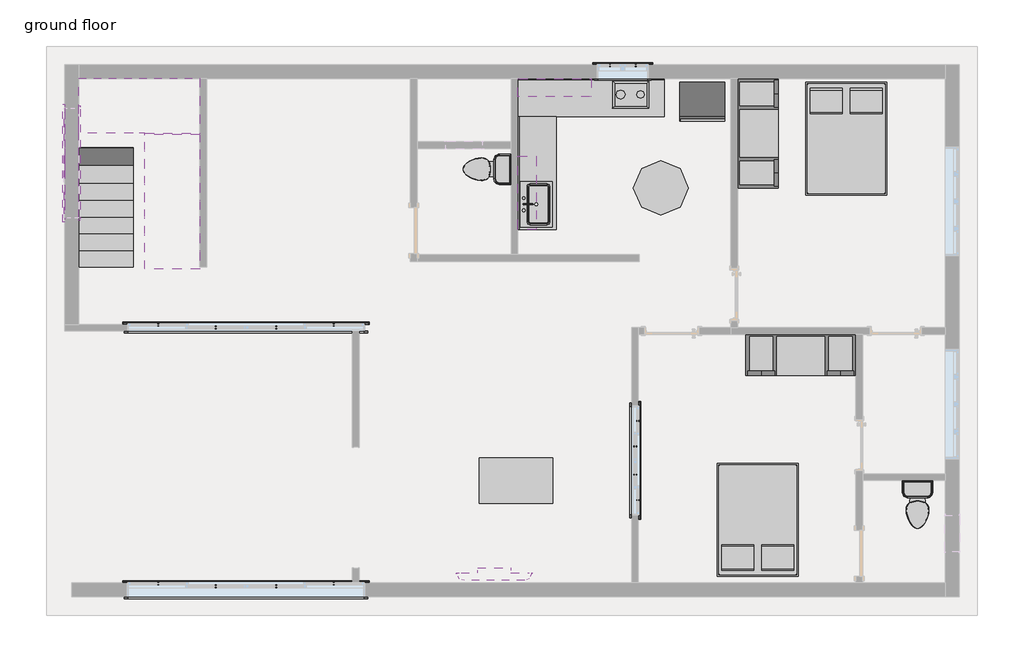
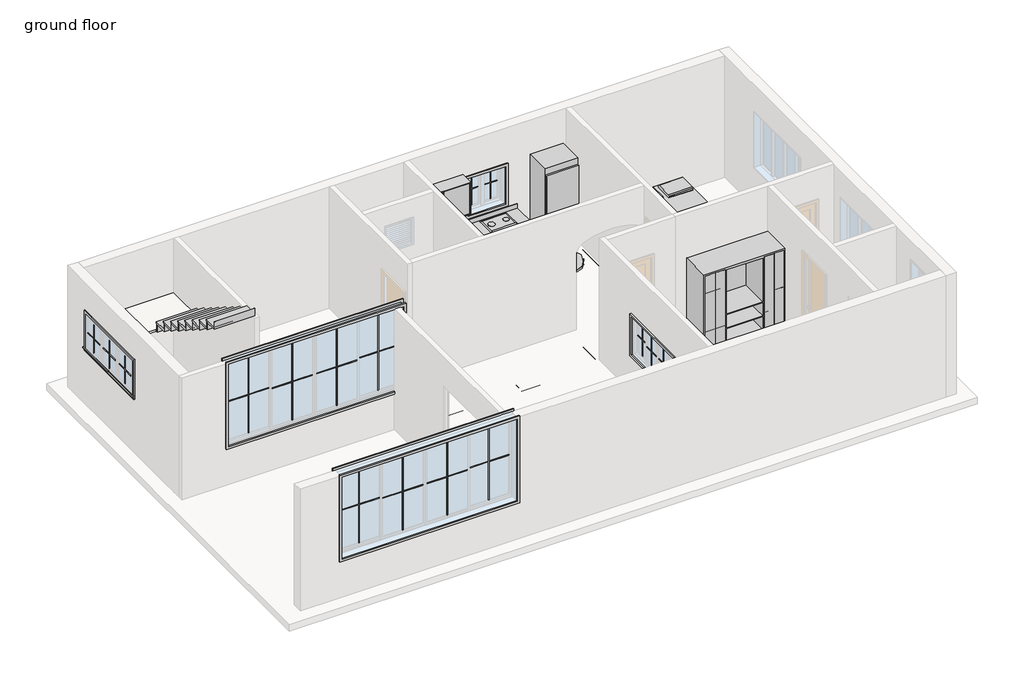
# One storey, part 2 of 2: 30 proxies, 15 furniture elements, 9 beams, 3 flow terminals, 2 stair flights, 1 slab.
"""IFC4 building model written with IfcOpenShell, lengths in millimetres."""

from ifc_helpers import new_model, si_unit, frame, origin, place, context, project, spatial, polyline, outline, extrude, faceted_brep, transform, mapped, element, save
from components import proxy_3c1fa1d0, proxy_caef4acf, muntin_pattern_2x2_muntin_pattern_2x2_31a16349, muntin_pattern_2x2_muntin_pattern_2x2_a56fcb99, muntin_pattern_2x2_muntin_pattern_2x2_c58f38d7, muntin_pattern_2x2_muntin_pattern_2x2_b3fe6957, muntin_pattern_2x2_muntin_pattern_2x2_3e0ecaf2, muntin_pattern_2x2_muntin_pattern_2x2_51cb8927, proxy_19935bb1, trim_window_exterior_flat_with_sill_3c945769, trim_window_exterior_flat_with_sill_7b949e88, trim_window_exterior_flat_with_sill_41619996, trim_window_exterior_flat_with_sill_170b7f0e, trim_window_interior_flat_picture_frame_0edfbaa2, trim_window_interior_flat_picture_frame_687edbe0, trim_window_interior_flat_picture_frame_51c85655, trim_window_interior_flat_picture_frame_cc79b2fe, flow_terminal_4d548711, toilet_domestic_3d_toilet_domestic_3d_ba6479b0, toilet_domestic_3d_toilet_domestic_3d_30431060, furniture_f87f75a4, furniture_97fe820d, furniture_b58f7881, furniture_deb1c5d1, furniture_078eb3f3, furniture_88072bd9, furniture_0b81fedb, furniture_acc2807d, furniture_52f35bf4, furniture_f491f192, non_monolithic_landing_2b816123, stair_flight_0432408d, stair_flight_b9007331

model = new_model("IFC4")

# Units and contexts
model_context = context("Model", 3, world=origin())
ifc_project = project(units=[si_unit("LENGTHUNIT", "METRE", prefix="MILLI")], contexts=[model_context])

# Site, building, storey
site = spatial("IfcSite", under=ifc_project)
building = spatial("IfcBuilding", under=site)
storey = spatial("IfcBuildingStorey", under=building, Name="ground floor", Elevation=609.6)

# Beams
placement = place(None, origin())
element("IfcBeam", 1, ObjectType="Concrete-Rectangular Beam", at=placement, inside=storey, context=model_context, shape_type="Brep", body=[
    faceted_brep([(-12643.368339, 9510.993496, 609.6), (-12643.368339, 9282.393496, 609.6), (-10681.218339, 9282.393496, 609.6), (-10452.618339, 9282.393496, 609.6), (-7176.018339, 9282.393496, 609.6), (-6947.418339, 9282.393496, 609.6), (-5499.618339, 9282.393496, 609.6), (-5271.018339, 9282.393496, 609.6), (-3492.916739, 9282.393496, 609.6), (-3264.316739, 9282.393496, 609.6), (-1842.018339, 9282.393496, 609.6), (-1613.418339, 9282.393496, 609.6), (1790.181661, 9282.393496, 609.6), (1790.181661, 9510.993496, 609.6), (-1575.318339, 9510.993496, 609.6), (-1575.318339, 9320.493496, 609.6), (-1880.118339, 9320.493496, 609.6), (-1880.118339, 9510.993496, 609.6), (-6909.318339, 9510.993496, 609.6), (-6909.318339, 9320.493496, 609.6), (-7214.118339, 9320.493496, 609.6), (-7214.118339, 9510.993496, 609.6), (-10414.518339, 9510.993496, 609.6), (-10414.518339, 9320.493496, 609.6), (-10719.318339, 9320.493496, 609.6), (-10719.318339, 9510.993496, 609.6), (-12643.368339, 9282.393496, 304.8), (-10681.218339, 9282.393496, 304.8), (-10452.618339, 9282.393496, 304.8), (-7176.018339, 9282.393496, 304.8), (-6947.418339, 9282.393496, 304.8), (-5499.618339, 9282.393496, 304.8), (-5271.018339, 9282.393496, 304.8), (-3492.916739, 9282.393496, 304.8), (-3264.316739, 9282.393496, 304.8), (-1842.018339, 9282.393496, 304.8), (-1613.418339, 9282.393496, 304.8), (1790.181661, 9282.393496, 304.8), (-12643.368339, 9510.993496, 304.8), (-10719.318339, 9510.993496, 304.8), (-10719.318339, 9320.493496, 304.8), (-10414.518339, 9320.493496, 304.8), (-10414.518339, 9510.993496, 304.8), (-7214.118339, 9510.993496, 304.8), (-7214.118339, 9320.493496, 304.8), (-6909.318339, 9320.493496, 304.8), (-6909.318339, 9510.993496, 304.8), (-1880.118339, 9510.993496, 304.8), (-1880.118339, 9320.493496, 304.8), (-1575.318339, 9320.493496, 304.8), (-1575.318339, 9510.993496, 304.8), (1790.181661, 9510.993496, 304.8)], [[[0, 1, 2, 3, 4, 5, 6, 7, 8, 9, 10, 11, 12, 13, 14, 15, 16, 17, 18, 19, 20, 21, 22, 23, 24, 25]], [[1, 26, 27, 28, 29, 30, 31, 32, 33, 34, 35, 36, 37, 12, 11, 10, 9, 8, 7, 6, 5, 4, 3, 2]], [[26, 38, 39, 40, 41, 42, 43, 44, 45, 46, 47, 48, 49, 50, 51, 37, 36, 35, 34, 33, 32, 31, 30, 29, 28, 27]], [[13, 51, 50, 14]], [[1, 0, 38, 26]], [[13, 12, 37, 51]], [[41, 23, 22, 42]], [[23, 41, 40, 24]], [[24, 40, 39, 25]], [[45, 19, 18, 46]], [[19, 45, 44, 20]], [[20, 44, 43, 21]], [[49, 15, 14, 50]], [[15, 49, 48, 16]], [[16, 48, 47, 17]], [[38, 0, 25, 39]], [[42, 22, 21, 43]], [[46, 18, 17, 47]]]),
])
element("IfcBeam", 2, ObjectType="Concrete-Rectangular Beam", at=placement, inside=storey, context=model_context, shape_type="Brep", body=[
    faceted_brep([(1790.181661, 913.093496, 609.6), (2018.781661, 913.093496, 609.6), (2018.781661, 4958.043496, 609.6), (1790.181661, 4958.043496, 609.6), (1790.181661, 2792.693496, 609.6), (1790.181661, 2564.093496, 609.6), (1790.181661, 913.093496, 304.8), (1790.181661, 4958.043496, 304.8), (1790.181661, 2792.693496, 304.8), (1790.181661, 2564.093496, 304.8), (2018.781661, 913.093496, 304.8), (2018.781661, 4958.043496, 304.8)], [[[0, 1, 2, 3, 4, 5]], [[6, 0, 5, 4, 3, 7, 8, 9]], [[10, 6, 9, 8, 7, 11]], [[1, 10, 11, 2]], [[1, 0, 6, 10]], [[3, 2, 11, 7]]]),
    faceted_brep([(1790.181661, 9244.293496, 609.6), (2018.781661, 9244.293496, 609.6), (2018.781661, 9244.293496, 304.8), (1790.181661, 9244.293496, 304.8), (2018.781661, 5262.843496, 609.6), (1790.181661, 5262.843496, 609.6), (1790.181661, 5262.843496, 304.8), (2018.781661, 5262.843496, 304.8), (1790.181661, 6443.943496, 609.6), (1790.181661, 6215.343496, 609.6), (1790.181661, 6443.943496, 304.8), (1790.181661, 6215.343496, 304.8)], [[[0, 1, 2, 3]], [[4, 5, 6, 7]], [[1, 0, 8, 9, 5, 4]], [[0, 3, 10, 11, 6, 5, 9, 8]], [[3, 2, 7, 6, 11, 10]], [[2, 1, 4, 7]]]),
])
element("IfcBeam", 3, ObjectType="Concrete-Rectangular Beam", at=placement, inside=storey, context=model_context, shape_type="SweptSolid", body=[
    extrude(outline(polyline([(-6947.418339, 8094.943496), (-6947.418339, 8323.543496), (-5499.618339, 8323.543496), (-5499.618339, 8094.943496), (-6947.418339, 8094.943496)])), frame((0.0, 0.0, 304.8), z_axis=(0.0, 0.0, 1.0), x_axis=(1.0, 0.0, 0.0)), (0.0, 0.0, 1.0), 304.8),
])
element("IfcBeam", 4, ObjectType="Concrete-Rectangular Beam", at=placement, inside=storey, context=model_context, shape_type="Brep", body=[
    faceted_brep([(-6947.418339, 6443.943496, 609.6), (-6947.418339, 6215.343496, 609.6), (-5499.618339, 6215.343496, 609.6), (-5499.618339, 6443.943496, 609.6), (-6947.418339, 6215.343496, 304.8), (-5499.618339, 6215.343496, 304.8), (-6947.418339, 6443.943496, 304.8), (-5499.618339, 6443.943496, 304.8)], [[[0, 1, 2, 3]], [[1, 4, 5, 2]], [[4, 6, 7, 5]], [[6, 0, 3, 7]], [[1, 0, 6, 4]], [[3, 2, 5, 7]]]),
    faceted_brep([(1790.181661, 6443.943496, 609.6), (1790.181661, 6215.343496, 609.6), (1790.181661, 6215.343496, 304.8), (1790.181661, 6443.943496, 304.8), (-5271.018339, 6215.343496, 609.6), (-5271.018339, 6443.943496, 609.6), (-5271.018339, 6443.943496, 304.8), (-5271.018339, 6215.343496, 304.8), (-1613.418339, 6443.943496, 609.6), (-1842.018339, 6443.943496, 609.6), (-3264.316739, 6443.943496, 609.6), (-3492.916739, 6443.943496, 609.6), (-3492.916739, 6215.343496, 609.6), (-3264.316739, 6215.343496, 609.6), (-1842.018339, 6215.343496, 609.6), (-1613.418339, 6215.343496, 609.6), (-3492.916739, 6215.343496, 304.8), (-3264.316739, 6215.343496, 304.8), (-1842.018339, 6215.343496, 304.8), (-1613.418339, 6215.343496, 304.8), (-3492.916739, 6443.943496, 304.8), (-3264.316739, 6443.943496, 304.8), (-1842.018339, 6443.943496, 304.8), (-1613.418339, 6443.943496, 304.8)], [[[0, 1, 2, 3]], [[4, 5, 6, 7]], [[1, 0, 8, 9, 10, 11, 5, 4, 12, 13, 14, 15]], [[2, 1, 15, 14, 13, 12, 4, 7, 16, 17, 18, 19]], [[3, 2, 19, 18, 17, 16, 7, 6, 20, 21, 22, 23]], [[0, 3, 23, 22, 21, 20, 6, 5, 11, 10, 9, 8]]]),
])
element("IfcBeam", 5, ObjectType="Concrete-Rectangular Beam", at=placement, inside=storey, context=model_context, shape_type="Brep", body=[
    faceted_brep([(-1842.018339, 913.093496, 609.6), (-1613.418339, 913.093496, 609.6), (-1613.418339, 4996.143496, 609.6), (-1613.418339, 5224.743496, 609.6), (-1613.418339, 6215.343496, 609.6), (-1842.018339, 6215.343496, 609.6), (-1842.018339, 5281.893496, 609.6), (-1784.868339, 5281.893496, 609.6), (-1784.868339, 5053.293496, 609.6), (-1842.018339, 5053.293496, 609.6), (-1842.018339, 4996.143496, 609.6), (-1842.018339, 913.093496, 304.8), (-1842.018339, 5053.293496, 304.8), (-1842.018339, 4996.143496, 304.8), (-1613.418339, 913.093496, 304.8), (-1784.868339, 5053.293496, 304.8), (-1784.868339, 5281.893496, 304.8), (-1842.018339, 5281.893496, 304.8), (-1842.018339, 6215.343496, 304.8), (-1613.418339, 6215.343496, 304.8), (-1613.418339, 5224.743496, 304.8), (-1613.418339, 4996.143496, 304.8)], [[[0, 1, 2, 3, 4, 5, 6, 7, 8, 9, 10]], [[11, 0, 10, 9, 12, 13]], [[14, 11, 13, 12, 15, 16, 17, 18, 19, 20, 21]], [[1, 14, 21, 20, 19, 4, 3, 2]], [[1, 0, 11, 14]], [[8, 15, 12, 9]], [[16, 7, 6, 17]], [[7, 16, 15, 8]], [[17, 6, 5, 18]], [[5, 4, 19, 18]]]),
    faceted_brep([(-1842.018339, 9282.393496, 609.6), (-1613.418339, 9282.393496, 609.6), (-1613.418339, 9282.393496, 304.8), (-1842.018339, 9282.393496, 304.8), (-1613.418339, 6443.943496, 609.6), (-1842.018339, 6443.943496, 609.6), (-1842.018339, 6443.943496, 304.8), (-1613.418339, 6443.943496, 304.8)], [[[0, 1, 2, 3]], [[4, 5, 6, 7]], [[1, 0, 5, 4]], [[3, 2, 7, 6]], [[2, 1, 4, 7]], [[0, 3, 6, 5]]]),
])
element("IfcBeam", 6, ObjectType="Concrete-Rectangular Beam", at=placement, inside=storey, context=model_context, shape_type="Brep", body=[
    faceted_brep([(-7912.618339, 5224.743496, 609.6), (-7912.618339, 5148.543496, 609.6), (-7912.618339, 4996.143496, 609.6), (-7176.018339, 4996.143496, 609.6), (-7176.018339, 5224.743496, 609.6), (-7912.618339, 5224.743496, 304.8), (-7176.018339, 5224.743496, 304.8), (-7912.618339, 4996.143496, 304.8), (-7912.618339, 5148.543496, 304.8), (-7176.018339, 4996.143496, 304.8)], [[[0, 1, 2, 3, 4]], [[5, 0, 4, 6]], [[7, 8, 5, 6, 9]], [[2, 7, 9, 3]], [[0, 5, 8, 7, 2, 1]], [[4, 3, 9, 6]]]),
    faceted_brep([(1790.181661, 5224.743496, 609.6), (1790.181661, 4996.143496, 609.6), (1790.181661, 4996.143496, 304.8), (1790.181661, 5224.743496, 304.8), (-1613.418339, 5224.743496, 304.8), (-1613.418339, 5224.743496, 609.6), (-1613.418339, 4996.143496, 304.8), (-1613.418339, 4996.143496, 609.6), (240.781661, 4996.143496, 609.6), (469.381661, 4996.143496, 609.6), (469.381661, 4996.143496, 304.8), (240.781661, 4996.143496, 304.8)], [[[0, 1, 2, 3]], [[0, 3, 4, 5]], [[5, 4, 6, 7]], [[1, 0, 5, 7, 8, 9]], [[3, 2, 10, 11, 6, 4]], [[2, 1, 9, 8, 7, 6, 11, 10]]]),
    faceted_brep([(-2089.668339, 5053.293496, 304.8), (-2089.668339, 5053.293496, 609.6), (-1842.018339, 5053.293496, 609.6), (-1842.018339, 5053.293496, 304.8), (-2089.668339, 5224.743496, 304.8), (-2089.668339, 5224.743496, 609.6), (-5271.018339, 4996.143496, 609.6), (-5271.018339, 5224.743496, 609.6), (-5271.018339, 5224.743496, 304.8), (-5271.018339, 4996.143496, 304.8), (-3264.316739, 5224.743496, 609.6), (-3492.916739, 5224.743496, 609.6), (-3492.916739, 4996.143496, 609.6), (-3264.316739, 4996.143496, 609.6), (-1842.018339, 4996.143496, 609.6), (-3264.316739, 5224.743496, 304.8), (-3492.916739, 5224.743496, 304.8), (-1842.018339, 4996.143496, 304.8), (-3264.316739, 4996.143496, 304.8), (-3492.916739, 4996.143496, 304.8)], [[[0, 1, 2, 3]], [[1, 0, 4, 5]], [[6, 7, 8, 9]], [[1, 5, 10, 11, 7, 6, 12, 13, 14, 2]], [[5, 4, 15, 16, 8, 7, 11, 10]], [[4, 0, 3, 17, 18, 19, 9, 8, 16, 15]], [[6, 9, 19, 18, 17, 14, 13, 12]], [[3, 2, 14, 17]]]),
    faceted_brep([(-6947.418339, 4996.143496, 609.6), (-6947.418339, 5224.743496, 609.6), (-6947.418339, 5224.743496, 304.8), (-6947.418339, 4996.143496, 304.8), (-5499.618339, 4996.143496, 609.6), (-5499.618339, 5224.743496, 609.6), (-5499.618339, 5224.743496, 304.8), (-5499.618339, 4996.143496, 304.8)], [[[0, 1, 2, 3]], [[1, 0, 4, 5]], [[2, 1, 5, 6]], [[3, 2, 6, 7]], [[0, 3, 7, 4]], [[5, 4, 7, 6]]]),
])
element("IfcBeam", 7, ObjectType="Concrete-Rectangular Beam", at=placement, inside=storey, context=model_context, shape_type="SweptSolid", body=[
    extrude(outline(polyline([(-3492.916739, 9282.393496), (-3264.316739, 9282.393496), (-3264.316739, 6443.943496), (-3492.916739, 6443.943496), (-3492.916739, 9282.393496)])), frame((0.0, 0.0, 304.8), z_axis=(0.0, 0.0, 1.0), x_axis=(1.0, 0.0, 0.0)), (0.0, 0.0, 1.0), 304.8),
    extrude(outline(polyline([(-3264.316739, 913.093496), (-3492.916739, 913.093496), (-3492.916739, 4996.143496), (-3264.316739, 4996.143496), (-3264.316739, 913.093496)])), frame((0.0, 0.0, 304.8), z_axis=(0.0, 0.0, 1.0), x_axis=(1.0, 0.0, 0.0)), (0.0, 0.0, 1.0), 304.8),
    extrude(outline(polyline([(-3492.916739, 6215.343496), (-3264.316739, 6215.343496), (-3264.316739, 5224.743496), (-3492.916739, 5224.743496), (-3492.916739, 6215.343496)])), frame((0.0, 0.0, 304.8), z_axis=(0.0, 0.0, 1.0), x_axis=(1.0, 0.0, 0.0)), (0.0, 0.0, 1.0), 304.8),
])
element("IfcBeam", 8, ObjectType="Concrete-Rectangular Beam", at=placement, inside=storey, context=model_context, shape_type="Brep", body=[
    faceted_brep([(240.781661, 913.093496, 609.6), (469.381661, 913.093496, 609.6), (469.381661, 2564.093496, 609.6), (469.381661, 2792.693496, 609.6), (469.381661, 4996.143496, 609.6), (240.781661, 4996.143496, 609.6), (469.381661, 913.093496, 304.8), (469.381661, 2564.093496, 304.8), (469.381661, 2792.693496, 304.8), (469.381661, 4996.143496, 304.8), (240.781661, 913.093496, 304.8), (240.781661, 4996.143496, 304.8)], [[[0, 1, 2, 3, 4, 5]], [[1, 6, 7, 8, 9, 4, 3, 2]], [[6, 10, 11, 9, 8, 7]], [[10, 0, 5, 11]], [[1, 0, 10, 6]], [[5, 4, 9, 11]]]),
])
element("IfcBeam", 9, ObjectType="Concrete-Rectangular Beam", at=placement, inside=storey, context=model_context, shape_type="SweptSolid", body=[
    extrude(outline(polyline([(1790.181661, 2792.693496), (1790.181661, 2564.093496), (469.381661, 2564.093496), (469.381661, 2792.693496), (1790.181661, 2792.693496)])), frame((0.0, 0.0, 304.8), z_axis=(0.0, 0.0, 1.0), x_axis=(1.0, 0.0, 0.0)), (0.0, 0.0, 1.0), 304.8),
])

# Proxies
proxy_shape = proxy_3c1fa1d0(model_context)
element("IfcBuildingElementProxy", 10, Name="Cook Top-2 Unit : 12\" x 18\"", ObjectType="Cook Top-2 Unit : 12\" x 18\"", at=placement, inside=storey, context=model_context, shape_type="MappedRepresentation", body=[
    mapped(proxy_shape, transform((-3421.5185434, 8977.593496, 609.6), x_axis=(0.0, 1.0, 0.0), y_axis=(-1.0, 0.0, 0.0), z_axis=(0.0, 0.0, 1.0))),
])
proxy_2_shape = proxy_caef4acf(model_context)
element("IfcBuildingElementProxy", 11, Name="Cook Top-2 Unit : 16\" x 22\"", ObjectType="Cook Top-2 Unit : 16\" x 22\"", at=placement, inside=storey, context=model_context, shape_type="MappedRepresentation", body=[
    mapped(proxy_2_shape, transform((-3370.7185434, 8977.593496, 609.6), x_axis=(0.0, 1.0, 0.0), y_axis=(-1.0, 0.0, 0.0), z_axis=(0.0, 0.0, 1.0))),
])
muntin_pattern_2x2_muntin_pattern_2x2_shape = muntin_pattern_2x2_muntin_pattern_2x2_31a16349(model_context)
element("IfcBuildingElementProxy", 12, Name="Muntin Pattern_2x2 : Muntin Pattern_2x2", ObjectType="Muntin Pattern_2x2 : Muntin Pattern_2x2", at=placement, inside=storey, context=model_context, shape_type="MappedRepresentation", body=[
    mapped(muntin_pattern_2x2_muntin_pattern_2x2_shape, transform((-3330.991739, 3615.018496, 1606.55), x_axis=(0.0, -1.0, 0.0), y_axis=(1.0, 0.0, 0.0), z_axis=(0.0, 0.0, 1.0))),
])
element("IfcBuildingElementProxy", 13, Name="Muntin Pattern_2x2 : Muntin Pattern_2x2", ObjectType="Muntin Pattern_2x2 : Muntin Pattern_2x2", at=placement, inside=storey, context=model_context, shape_type="MappedRepresentation", body=[
    mapped(muntin_pattern_2x2_muntin_pattern_2x2_shape, transform((-3375.441739, 3189.568496, 1606.55), x_axis=(0.0, -1.0, 0.0), y_axis=(1.0, 0.0, 0.0), z_axis=(0.0, 0.0, 1.0))),
])
element("IfcBuildingElementProxy", 14, Name="Muntin Pattern_2x2 : Muntin Pattern_2x2", ObjectType="Muntin Pattern_2x2 : Muntin Pattern_2x2", at=placement, inside=storey, context=model_context, shape_type="MappedRepresentation", body=[
    mapped(muntin_pattern_2x2_muntin_pattern_2x2_shape, transform((-3375.441739, 2719.668496, 1606.55), x_axis=(0.0, -1.0, 0.0), y_axis=(1.0, 0.0, 0.0), z_axis=(0.0, 0.0, 1.0))),
])
element("IfcBuildingElementProxy", 15, Name="Muntin Pattern_2x2 : Muntin Pattern_2x2", ObjectType="Muntin Pattern_2x2 : Muntin Pattern_2x2", at=placement, inside=storey, context=model_context, shape_type="MappedRepresentation", body=[
    mapped(muntin_pattern_2x2_muntin_pattern_2x2_shape, transform((-3330.991739, 2294.218496, 1606.55), x_axis=(0.0, -1.0, 0.0), y_axis=(1.0, 0.0, 0.0), z_axis=(0.0, 0.0, 1.0))),
])
muntin_pattern_2x2_muntin_pattern_2x2_2_shape = muntin_pattern_2x2_muntin_pattern_2x2_a56fcb99(model_context)
element("IfcBuildingElementProxy", 16, Name="Muntin Pattern_2x2 : Muntin Pattern_2x2", ObjectType="Muntin Pattern_2x2 : Muntin Pattern_2x2", at=placement, inside=storey, context=model_context, shape_type="MappedRepresentation", body=[
    mapped(muntin_pattern_2x2_muntin_pattern_2x2_2_shape, transform((-12862.443339, 7303.3101627, 2051.05), x_axis=(0.0, 1.0, 0.0), y_axis=(-1.0, 0.0, 0.0), z_axis=(0.0, 0.0, 1.0))),
])
element("IfcBuildingElementProxy", 17, Name="Muntin Pattern_2x2 : Muntin Pattern_2x2", ObjectType="Muntin Pattern_2x2 : Muntin Pattern_2x2", at=placement, inside=storey, context=model_context, shape_type="MappedRepresentation", body=[
    mapped(muntin_pattern_2x2_muntin_pattern_2x2_2_shape, transform((-12862.443339, 7910.793496, 2051.05), x_axis=(0.0, 1.0, 0.0), y_axis=(-1.0, 0.0, 0.0), z_axis=(0.0, 0.0, 1.0))),
])
muntin_pattern_2x2_muntin_pattern_2x2_3_shape = muntin_pattern_2x2_muntin_pattern_2x2_c58f38d7(model_context)
element("IfcBuildingElementProxy", 18, Name="Muntin Pattern_2x2 : Muntin Pattern_2x2", ObjectType="Muntin Pattern_2x2 : Muntin Pattern_2x2", at=placement, inside=storey, context=model_context, shape_type="MappedRepresentation", body=[
    mapped(muntin_pattern_2x2_muntin_pattern_2x2_3_shape, transform((-12862.443339, 8518.2768293, 2051.05), x_axis=(0.0, -1.0, 0.0), y_axis=(1.0, 0.0, 0.0), z_axis=(0.0, 0.0, 1.0))),
])
muntin_pattern_2x2_muntin_pattern_2x2_4_shape = muntin_pattern_2x2_muntin_pattern_2x2_b3fe6957(model_context)
element("IfcBuildingElementProxy", 19, Name="Muntin Pattern_2x2 : Muntin Pattern_2x2", ObjectType="Muntin Pattern_2x2 : Muntin Pattern_2x2", at=placement, inside=storey, context=model_context, shape_type="MappedRepresentation", body=[
    mapped(muntin_pattern_2x2_muntin_pattern_2x2_4_shape, transform((-3796.230839, 9539.568496, 1784.35), x_axis=(1.0, 0.0, 0.0), y_axis=(0.0, 1.0, 0.0), z_axis=(0.0, 0.0, 1.0))),
])
muntin_pattern_2x2_muntin_pattern_2x2_5_shape = muntin_pattern_2x2_muntin_pattern_2x2_3e0ecaf2(model_context)
element("IfcBuildingElementProxy", 20, Name="Muntin Pattern_2x2 : Muntin Pattern_2x2", ObjectType="Muntin Pattern_2x2 : Muntin Pattern_2x2", at=placement, inside=storey, context=model_context, shape_type="MappedRepresentation", body=[
    mapped(muntin_pattern_2x2_muntin_pattern_2x2_5_shape, transform((-3367.605839, 9539.568496, 1784.35), x_axis=(-1.0, 0.0, 0.0), y_axis=(0.0, -1.0, 0.0), z_axis=(0.0, 0.0, 1.0))),
])
muntin_pattern_2x2_muntin_pattern_2x2_6_shape = muntin_pattern_2x2_muntin_pattern_2x2_51cb8927(model_context)
element("IfcBuildingElementProxy", 21, Name="Muntin Pattern_2x2 : Muntin Pattern_2x2", ObjectType="Muntin Pattern_2x2 : Muntin Pattern_2x2", at=placement, inside=storey, context=model_context, shape_type="MappedRepresentation", body=[
    mapped(muntin_pattern_2x2_muntin_pattern_2x2_6_shape, transform((-11316.218339, 5215.218496, 1606.55), x_axis=(1.0, 0.0, 0.0), y_axis=(0.0, 1.0, 0.0), z_axis=(0.0, 0.0, 1.0))),
])
element("IfcBuildingElementProxy", 22, Name="Muntin Pattern_2x2 : Muntin Pattern_2x2", ObjectType="Muntin Pattern_2x2 : Muntin Pattern_2x2", at=placement, inside=storey, context=model_context, shape_type="MappedRepresentation", body=[
    mapped(muntin_pattern_2x2_muntin_pattern_2x2_6_shape, transform((-10357.368339, 5170.768496, 1606.55), x_axis=(1.0, 0.0, 0.0), y_axis=(0.0, 1.0, 0.0), z_axis=(0.0, 0.0, 1.0))),
])
element("IfcBuildingElementProxy", 23, Name="Muntin Pattern_2x2 : Muntin Pattern_2x2", ObjectType="Muntin Pattern_2x2 : Muntin Pattern_2x2", at=placement, inside=storey, context=model_context, shape_type="MappedRepresentation", body=[
    mapped(muntin_pattern_2x2_muntin_pattern_2x2_6_shape, transform((-9354.068339, 5170.768496, 1606.55), x_axis=(1.0, 0.0, 0.0), y_axis=(0.0, 1.0, 0.0), z_axis=(0.0, 0.0, 1.0))),
])
element("IfcBuildingElementProxy", 24, Name="Muntin Pattern_2x2 : Muntin Pattern_2x2", ObjectType="Muntin Pattern_2x2 : Muntin Pattern_2x2", at=placement, inside=storey, context=model_context, shape_type="MappedRepresentation", body=[
    mapped(muntin_pattern_2x2_muntin_pattern_2x2_6_shape, transform((-8395.218339, 5215.218496, 1606.55), x_axis=(1.0, 0.0, 0.0), y_axis=(0.0, 1.0, 0.0), z_axis=(0.0, 0.0, 1.0))),
])
element("IfcBuildingElementProxy", 25, Name="Muntin Pattern_2x2 : Muntin Pattern_2x2", ObjectType="Muntin Pattern_2x2 : Muntin Pattern_2x2", at=placement, inside=storey, context=model_context, shape_type="MappedRepresentation", body=[
    mapped(muntin_pattern_2x2_muntin_pattern_2x2_6_shape, transform((-11316.218339, 903.568496, 1606.55), x_axis=(1.0, 0.0, 0.0), y_axis=(0.0, 1.0, 0.0), z_axis=(0.0, 0.0, 1.0))),
])
element("IfcBuildingElementProxy", 26, Name="Muntin Pattern_2x2 : Muntin Pattern_2x2", ObjectType="Muntin Pattern_2x2 : Muntin Pattern_2x2", at=placement, inside=storey, context=model_context, shape_type="MappedRepresentation", body=[
    mapped(muntin_pattern_2x2_muntin_pattern_2x2_6_shape, transform((-10357.368339, 859.118496, 1606.55), x_axis=(1.0, 0.0, 0.0), y_axis=(0.0, 1.0, 0.0), z_axis=(0.0, 0.0, 1.0))),
])
element("IfcBuildingElementProxy", 27, Name="Muntin Pattern_2x2 : Muntin Pattern_2x2", ObjectType="Muntin Pattern_2x2 : Muntin Pattern_2x2", at=placement, inside=storey, context=model_context, shape_type="MappedRepresentation", body=[
    mapped(muntin_pattern_2x2_muntin_pattern_2x2_6_shape, transform((-9354.068339, 859.118496, 1606.55), x_axis=(1.0, 0.0, 0.0), y_axis=(0.0, 1.0, 0.0), z_axis=(0.0, 0.0, 1.0))),
])
element("IfcBuildingElementProxy", 28, Name="Muntin Pattern_2x2 : Muntin Pattern_2x2", ObjectType="Muntin Pattern_2x2 : Muntin Pattern_2x2", at=placement, inside=storey, context=model_context, shape_type="MappedRepresentation", body=[
    mapped(muntin_pattern_2x2_muntin_pattern_2x2_6_shape, transform((-8395.218339, 903.568496, 1606.55), x_axis=(1.0, 0.0, 0.0), y_axis=(0.0, 1.0, 0.0), z_axis=(0.0, 0.0, 1.0))),
])
proxy_3_shape = proxy_19935bb1(model_context)
element("IfcBuildingElementProxy", 29, Name="Refrigerator-Built-in : 30\" x 24\" LH", ObjectType="Refrigerator-Built-in : 30\" x 24\" LH", at=placement, inside=storey, context=model_context, shape_type="MappedRepresentation", body=[
    mapped(proxy_3_shape, transform((-2254.768339, 8966.8695245, 609.6), x_axis=(1.0, 0.0, 0.0), y_axis=(0.0, 1.0, 0.0), z_axis=(0.0, 0.0, 1.0))),
])
trim_window_exterior_flat_with_sill_shape = trim_window_exterior_flat_with_sill_3c945769(model_context)
element("IfcBuildingElementProxy", 30, Name="Trim-Window-Exterior-Flat : with Sill", ObjectType="Trim-Window-Exterior-Flat : with Sill", at=placement, inside=storey, context=model_context, shape_type="MappedRepresentation", body=[
    mapped(trim_window_exterior_flat_with_sill_shape, transform((-3321.466739, 2954.618496, 2438.4), x_axis=(0.0, 1.0, 0.0), y_axis=(0.0, 0.0, 1.0), z_axis=(1.0, 0.0, 0.0))),
])
trim_window_exterior_flat_with_sill_2_shape = trim_window_exterior_flat_with_sill_7b949e88(model_context)
element("IfcBuildingElementProxy", 31, Name="Trim-Window-Exterior-Flat : with Sill", ObjectType="Trim-Window-Exterior-Flat : with Sill", at=placement, inside=storey, context=model_context, shape_type="MappedRepresentation", body=[
    mapped(trim_window_exterior_flat_with_sill_2_shape, transform((-12871.968339, 7910.793496, 2794.0), x_axis=(0.0, 1.0, 0.0), y_axis=(0.0, 0.0, -1.0), z_axis=(-1.0, 0.0, 0.0))),
])
trim_window_exterior_flat_with_sill_3_shape = trim_window_exterior_flat_with_sill_41619996(model_context)
element("IfcBuildingElementProxy", 32, Name="Trim-Window-Exterior-Flat : with Sill", ObjectType="Trim-Window-Exterior-Flat : with Sill", at=placement, inside=storey, context=model_context, shape_type="MappedRepresentation", body=[
    mapped(trim_window_exterior_flat_with_sill_3_shape, transform((-3581.918339, 9549.093496, 2628.9), x_axis=(-1.0, 0.0, 0.0), y_axis=(0.0, 0.0, 1.0), z_axis=(0.0, 1.0, 0.0))),
])
trim_window_exterior_flat_with_sill_4_shape = trim_window_exterior_flat_with_sill_170b7f0e(model_context)
element("IfcBuildingElementProxy", 33, Name="Trim-Window-Exterior-Flat : with Sill", ObjectType="Trim-Window-Exterior-Flat : with Sill", at=placement, inside=storey, context=model_context, shape_type="MappedRepresentation", body=[
    mapped(trim_window_exterior_flat_with_sill_4_shape, transform((-9855.718339, 5224.743496, 3505.2), x_axis=(-1.0, 0.0, 0.0), y_axis=(0.0, 0.0, 1.0), z_axis=(0.0, 1.0, 0.0))),
])
element("IfcBuildingElementProxy", 34, Name="Trim-Window-Exterior-Flat : with Sill", ObjectType="Trim-Window-Exterior-Flat : with Sill", at=placement, inside=storey, context=model_context, shape_type="MappedRepresentation", body=[
    mapped(trim_window_exterior_flat_with_sill_4_shape, transform((-9855.718339, 913.093496, 3505.2), x_axis=(-1.0, 0.0, 0.0), y_axis=(0.0, 0.0, 1.0), z_axis=(0.0, 1.0, 0.0))),
])
trim_window_interior_flat_picture_frame_shape = trim_window_interior_flat_picture_frame_0edfbaa2(model_context)
element("IfcBuildingElementProxy", 35, Name="Trim-Window-Interior-Flat : Picture Frame", ObjectType="Trim-Window-Interior-Flat : Picture Frame", at=placement, inside=storey, context=model_context, shape_type="MappedRepresentation", body=[
    mapped(trim_window_interior_flat_picture_frame_shape, transform((-3435.766739, 2954.618496, 2438.4), x_axis=(0.0, -1.0, 0.0), y_axis=(0.0, 0.0, 1.0), z_axis=(-1.0, 0.0, 0.0))),
])
trim_window_interior_flat_picture_frame_2_shape = trim_window_interior_flat_picture_frame_687edbe0(model_context)
element("IfcBuildingElementProxy", 36, Name="Trim-Window-Interior-Flat : Picture Frame", ObjectType="Trim-Window-Interior-Flat : Picture Frame", at=placement, inside=storey, context=model_context, shape_type="MappedRepresentation", body=[
    mapped(trim_window_interior_flat_picture_frame_2_shape, transform((-12643.368339, 7910.793496, 2794.0), x_axis=(0.0, -1.0, 0.0), y_axis=(0.0, 0.0, -1.0), z_axis=(1.0, 0.0, 0.0))),
])
trim_window_interior_flat_picture_frame_3_shape = trim_window_interior_flat_picture_frame_51c85655(model_context)
element("IfcBuildingElementProxy", 37, Name="Trim-Window-Interior-Flat : Picture Frame", ObjectType="Trim-Window-Interior-Flat : Picture Frame", at=placement, inside=storey, context=model_context, shape_type="MappedRepresentation", body=[
    mapped(trim_window_interior_flat_picture_frame_3_shape, transform((-3581.918339, 9320.493496, 2628.9), x_axis=(1.0, 0.0, 0.0), y_axis=(0.0, 0.0, 1.0), z_axis=(0.0, -1.0, 0.0))),
])
trim_window_interior_flat_picture_frame_4_shape = trim_window_interior_flat_picture_frame_cc79b2fe(model_context)
element("IfcBuildingElementProxy", 38, Name="Trim-Window-Interior-Flat : Picture Frame", ObjectType="Trim-Window-Interior-Flat : Picture Frame", at=placement, inside=storey, context=model_context, shape_type="MappedRepresentation", body=[
    mapped(trim_window_interior_flat_picture_frame_4_shape, transform((-9855.718339, 5110.443496, 3505.2), x_axis=(1.0, 0.0, 0.0), y_axis=(0.0, 0.0, 1.0), z_axis=(0.0, -1.0, 0.0))),
])
element("IfcBuildingElementProxy", 39, Name="Trim-Window-Interior-Flat : Picture Frame", ObjectType="Trim-Window-Interior-Flat : Picture Frame", at=placement, inside=storey, context=model_context, shape_type="MappedRepresentation", body=[
    mapped(trim_window_interior_flat_picture_frame_4_shape, transform((-9855.718339, 684.493496, 3505.2), x_axis=(1.0, 0.0, 0.0), y_axis=(0.0, 0.0, 1.0), z_axis=(0.0, -1.0, 0.0))),
])

# Flow terminals
flow_terminal_shape = flow_terminal_4d548711(model_context)
element("IfcFlowTerminal", 40, ObjectType="Sink Kitchen-Single : 30\" x 21\"", at=placement, inside=storey, context=model_context, shape_type="MappedRepresentation", body=[
    mapped(flow_terminal_shape, transform((-5021.0229378, 7209.3042554, 609.6), x_axis=(0.0, 1.0, 0.0), y_axis=(-1.0, 0.0, 0.0), z_axis=(0.0, 0.0, 1.0))),
])
toilet_domestic_3d_toilet_domestic_3d_shape = toilet_domestic_3d_toilet_domestic_3d_ba6479b0(model_context)
toilet_domestic_3d_toilet_domestic_3d_2_shape = toilet_domestic_3d_toilet_domestic_3d_30431060(model_context)
element("IfcFlowTerminal", 41, ObjectType="Toilet-Domestic-3D : Toilet-Domestic-3D", at=placement, inside=storey, context=model_context, shape_type="MappedRepresentation", body=[
    mapped(toilet_domestic_3d_toilet_domestic_3d_shape, transform((-5937.1643663, 7809.6710196, 609.6), x_axis=(0.0, -1.0, 0.0), y_axis=(1.0, 0.0, 0.0), z_axis=(0.0, 0.0, 1.0))),
    mapped(toilet_domestic_3d_toilet_domestic_3d_2_shape, transform((-5937.1643663, 7809.6710196, 609.6), x_axis=(0.0, -1.0, 0.0), y_axis=(1.0, 0.0, 0.0), z_axis=(0.0, 0.0, 1.0))),
])
element("IfcFlowTerminal", 42, ObjectType="Toilet-Domestic-3D : Toilet-Domestic-3D", at=placement, inside=storey, context=model_context, shape_type="MappedRepresentation", body=[
    mapped(toilet_domestic_3d_toilet_domestic_3d_shape, transform((1325.531896, 2126.5474686, 609.6), x_axis=(1.0, 0.0, 0.0), y_axis=(0.0, 1.0, 0.0), z_axis=(0.0, 0.0, 1.0))),
    mapped(toilet_domestic_3d_toilet_domestic_3d_2_shape, transform((1325.531896, 2126.5474686, 609.6), x_axis=(1.0, 0.0, 0.0), y_axis=(0.0, 1.0, 0.0), z_axis=(0.0, 0.0, 1.0))),
])

# Furniture
furniture_shape = furniture_f87f75a4(model_context)
element("IfcFurniture", 43, ObjectType="Base Cabinet-Combo01 : 30\"", at=placement, inside=storey, context=model_context, shape_type="MappedRepresentation", body=[
    mapped(furniture_shape, transform((-4051.5060439, 9320.493496, 609.6), x_axis=(1.0, 0.0, 0.0), y_axis=(0.0, 1.0, 0.0), z_axis=(0.0, 0.0, 1.0))),
])
element("IfcFurniture", 44, ObjectType="Base Cabinet-Combo01 : 30\"", at=placement, inside=storey, context=model_context, shape_type="MappedRepresentation", body=[
    mapped(furniture_shape, transform((-5328.168339, 8006.3557911, 609.6), x_axis=(0.0, 1.0, 0.0), y_axis=(-1.0, 0.0, 0.0), z_axis=(0.0, 0.0, 1.0))),
])
element("IfcFurniture", 45, ObjectType="Base Cabinet-Combo01 : 30\"", at=placement, inside=storey, context=model_context, shape_type="MappedRepresentation", body=[
    mapped(furniture_shape, transform((-3289.5060439, 9320.493496, 609.6), x_axis=(1.0, 0.0, 0.0), y_axis=(0.0, 1.0, 0.0), z_axis=(0.0, 0.0, 1.0))),
])
furniture_2_shape = furniture_97fe820d(model_context)
element("IfcFurniture", 46, ObjectType="Base Cabinet-Corner Unit-Square : 36\"", at=placement, inside=storey, context=model_context, shape_type="MappedRepresentation", body=[
    mapped(furniture_2_shape, transform((-5328.168339, 8793.7557911, 609.6), x_axis=(0.0, 1.0, 0.0), y_axis=(-1.0, 0.0, 0.0), z_axis=(0.0, 0.0, 1.0))),
])
furniture_3_shape = furniture_b58f7881(model_context)
element("IfcFurniture", 47, ObjectType="Bed-Box : Double 53\" x 74\"", at=placement, inside=storey, context=model_context, shape_type="MappedRepresentation", body=[
    mapped(furniture_3_shape, transform((-199.970798, 8551.6230042, 609.6), x_axis=(1.0, 0.0, 0.0), y_axis=(0.0, 1.0, 0.0), z_axis=(0.0, 0.0, 1.0))),
])
element("IfcFurniture", 48, ObjectType="Bed-Box : Double 53\" x 74\"", at=placement, inside=storey, context=model_context, shape_type="MappedRepresentation", body=[
    mapped(furniture_3_shape, transform((-994.7642799, 1732.7639878, 609.6), x_axis=(-1.0, 0.0, 0.0), y_axis=(0.0, -1.0, 0.0), z_axis=(0.0, 0.0, 1.0))),
])
furniture_4_shape = furniture_deb1c5d1(model_context)
element("IfcFurniture", 49, ObjectType="Counter Top : 24\" Depth", at=placement, inside=storey, context=model_context, shape_type="MappedRepresentation", body=[
    mapped(furniture_4_shape, transform((-4127.7060439, 9320.493496, 609.6), x_axis=(1.0, 0.0, 0.0), y_axis=(0.0, 1.0, 0.0), z_axis=(0.0, 0.0, 1.0))),
])
furniture_5_shape = furniture_078eb3f3(model_context)
element("IfcFurniture", 50, ObjectType="Counter Top w Sink Hole : 24\" Depth", at=placement, inside=storey, context=model_context, shape_type="MappedRepresentation", body=[
    mapped(furniture_5_shape, transform((-5328.168339, 8006.6364215, 609.6), x_axis=(0.0, 1.0, 0.0), y_axis=(-1.0, 0.0, 0.0), z_axis=(0.0, 0.0, 1.0))),
])
furniture_6_shape = furniture_88072bd9(model_context)
element("IfcFurniture", 51, ObjectType="Entertainment Center.0001 : 72\" x 72\" x 24\"", at=placement, inside=storey, context=model_context, shape_type="MappedRepresentation", body=[
    mapped(furniture_6_shape, transform((-616.468339, 5154.893496, 609.6), x_axis=(1.0, 0.0, 0.0), y_axis=(0.0, 1.0, 0.0), z_axis=(0.0, 0.0, 1.0))),
])
element("IfcFurniture", 52, ObjectType="Entertainment Center.0001 : 72\" x 72\" x 24\"", at=placement, inside=storey, context=model_context, shape_type="MappedRepresentation", body=[
    mapped(furniture_6_shape, transform((-1772.168339, 8406.093496, 609.6), x_axis=(0.0, 1.0, 0.0), y_axis=(-1.0, 0.0, 0.0), z_axis=(0.0, 0.0, 1.0))),
])
furniture_7_shape = furniture_0b81fedb(model_context)
element("IfcFurniture", 53, ObjectType="TV - Flat Screen : 50\"", at=placement, inside=storey, context=model_context, shape_type="MappedRepresentation", body=[
    mapped(furniture_7_shape, transform((-5725.8128531, 1013.6142575, 1828.8), x_axis=(-1.0, 0.0, 0.0), y_axis=(0.0, -1.0, 0.0), z_axis=(0.0, 0.0, 1.0))),
])
furniture_8_shape = furniture_acc2807d(model_context)
element("IfcFurniture", 54, ObjectType="Table-Coffee Rectangular : 48\" x 30\"", at=placement, inside=storey, context=model_context, shape_type="MappedRepresentation", body=[
    mapped(furniture_8_shape, transform((-5973.1503692, 2251.6326642, 609.6), x_axis=(1.0, 0.0, 0.0), y_axis=(0.0, 1.0, 0.0), z_axis=(0.0, 0.0, 1.0))),
])
furniture_9_shape = furniture_52f35bf4(model_context)
element("IfcFurniture", 55, ObjectType="Table-Dining Round w Chairs : 36\" Diameter", at=placement, inside=storey, context=model_context, shape_type="MappedRepresentation", body=[
    mapped(furniture_9_shape, transform((-3050.6003062, 7682.9221845, 609.6), x_axis=(1.0, 0.0, 0.0), y_axis=(0.0, 1.0, 0.0), z_axis=(0.0, 0.0, 1.0))),
])
furniture_10_shape = furniture_f491f192(model_context)
element("IfcFurniture", 56, ObjectType="Upper Cabinet-Pass-Thru w Glass : 48\" x 30\" x 12\"", at=placement, inside=storey, context=model_context, shape_type="MappedRepresentation", body=[
    mapped(furniture_10_shape, transform((-4737.3060439, 9320.493496, 609.6), x_axis=(1.0, 0.0, 0.0), y_axis=(0.0, 1.0, 0.0), z_axis=(0.0, 0.0, 1.0))),
])
element("IfcFurniture", 57, ObjectType="Upper Cabinet-Pass-Thru w Glass : 48\" x 30\" x 12\"", at=placement, inside=storey, context=model_context, shape_type="MappedRepresentation", body=[
    mapped(furniture_10_shape, transform((-5328.168339, 7397.0364215, 609.6), x_axis=(0.0, 1.0, 0.0), y_axis=(-1.0, 0.0, 0.0), z_axis=(0.0, 0.0, 1.0))),
])

# Slab
non_monolithic_landing_shape = non_monolithic_landing_2b816123(model_context)
element("IfcSlab", 58, ObjectType="Non-Monolithic Landing", at=placement, inside=storey, context=model_context, shape_type="MappedRepresentation", body=[
    mapped(non_monolithic_landing_shape, transform((0.0, 0.0, 0.0), x_axis=(1.0, 0.0, 0.0), y_axis=(0.0, 1.0, 0.0), z_axis=(0.0, 0.0, 1.0))),
])

# Stair flights
stair_flight_shape = stair_flight_0432408d(model_context)
element("IfcStairFlight", 59, ObjectType="2\" Tread 1\" Nosing 1/4\" Riser", at=placement, inside=storey, context=model_context, shape_type="MappedRepresentation", body=[
    mapped(stair_flight_shape, transform((0.0, 0.0, 0.0), x_axis=(1.0, 0.0, 0.0), y_axis=(0.0, 1.0, 0.0), z_axis=(0.0, 0.0, 1.0))),
])
stair_flight_2_shape = stair_flight_b9007331(model_context)
element("IfcStairFlight", 60, ObjectType="2\" Tread 1\" Nosing 1/4\" Riser", at=placement, inside=storey, context=model_context, shape_type="MappedRepresentation", body=[
    mapped(stair_flight_2_shape, transform((0.0, 0.0, 0.0), x_axis=(1.0, 0.0, 0.0), y_axis=(0.0, 1.0, 0.0), z_axis=(0.0, 0.0, 1.0))),
])

save(model, "model.ifc")

# Revit data of these elements
# Type "Concrete-Rectangular Beam"
#   Assembly Code = "B10"
#   Length [instance default] = 5 ft
#   b = 0.75 ft
#   h = 1 ft
#   Structural Material [instance default] = Concrete, Cast-in-Place gray
# Type "Cook Top-2 Unit : 12\" x 18\""
#   Assembly Code = "E1090400"
#   Counter Height = 3 ft
#   Depth = 2 ft
#   Width = 1.5 ft
#   Burner Material = Metal - Chrome
#   Cooktop Material = Metal - Steel, Polished
#   Default Elevation = 0
# Type "Cook Top-2 Unit : 16\" x 22\""
#   Assembly Code = "E1090400"
#   Counter Height = 2.583333 ft
#   Depth = 1.833333 ft
#   Width = 1.333333 ft
#   Burner Material = Metal - Chrome
#   Cooktop Material = Metal - Steel, Polished
#   Default Elevation = 0
# Type "Muntin Pattern_2x2 : Muntin Pattern_2x2"
#   Width [instance default] = 4 ft
#   Thickness = 0.041667 ft
#   Height [instance default] = 4 ft
#   Distance = 0.0625 ft
#   Interior Material [instance default] = none
#   Exterior Material [instance default] = none
#   Default Elevation = 0
# Type "Refrigerator-Built-in : 30\" x 24\" LH"
#   Assembly Code = "E1090400"
#   Depth = 2 ft
#   Handle = 0.020833 ft
#   Height = 7 ft
#   Top Door Height = 5 ft
#   Width = 2.458333 ft
#   Material = Metal - Paint Finish - Ivory,Glossy
#   Default Elevation = 0
# Type "Trim-Window-Exterior-Flat : with Sill"
#   Trim Width = 0.1875 ft
#   Trim Thickness_Picture Frame = 0.104167 ft
#   Trim Thickness_with Sill = 0.0625 ft
#   Sill Thickness = 0.104167 ft
#   Opening Width [instance default] = 2 ft
#   Opening Height [instance default] = 3 ft
#   Default Elevation = 4 ft
#   Sill = yes
#   Picture Frame = no
#   Trim Material [instance default] = none
# Type "Trim-Window-Interior-Flat : Picture Frame"
#   Trim Thickness_Picture Frame = 0.104167 ft
#   Trim Width = 0.1875 ft
#   Trim Thickness_with Sill = 0.0625 ft
#   Sill Thickness = 0.104167 ft
#   Opening Width [instance default] = 2 ft
#   Opening Height [instance default] = 3 ft
#   Default Elevation = 4 ft
#   Sill = no
#   Picture Frame = yes
#   Trim Material [instance default] = none
# Type "Sink Kitchen-Single : 30\" x 21\""
#   Assembly Code = "D2010410"
#   Counter Height = 3 ft
#   Depth = 1.75 ft
#   Width = 2.5 ft
#   Faucet Material = Steel, Polished
#   Sink Material = Steel, Polished
#   Default Elevation = 0
# Type "Toilet-Domestic-3D : Toilet-Domestic-3D"
#   Assembly Code = "D2010110"
#   Toilet - Bowl/Basin Material = Porcelain, Linen
#   Toilet - Seat Material = Laminate, Linen, Matte
#   Default Elevation = 0
# Type "Base Cabinet-Combo01 : 30\""
#   Depth = 1.833333 ft
#   Height = 2.979167 ft
#   Toe Depth = 0.25 ft
#   Toe Height = 0.291667 ft
#   Width = 2.5 ft
#   Default Elevation = 0
# Type "Base Cabinet-Corner Unit-Square : 36\""
#   Assembly Code = "C1030410"
#   Depth = 2 ft
#   Height = 2.875 ft
#   Toe Depth = 0.25 ft
#   Toe Height = 0.291667 ft
#   Width = 3 ft
#   Cabinet Material = Cabinets
#   Door/Drawer Material = Cabinets
#   Handle Material = Cabinets - Handles
#   Default Elevation = 0
# Type "Bed-Box : Double 53\" x 74\""
#   Assembly Code = "E2020200"
#   Length = 6.166667 ft
#   Width = 4.416667 ft
#   Frame Material = Birch
#   Mattress Material = Linen, White
#   Default Elevation = 0
# Type "Counter Top : 24\" Depth"
#   Assembly Code = "C1030400"
#   Counter Thickness = 0.125 ft
#   Depth = 2.083333 ft
#   Height = 3 ft
#   Length [instance default] = 8 ft
#   Counter Top Material = none
#   Default Elevation = 0
# Type "Counter Top w Sink Hole : 24\" Depth"
#   Assembly Code = "C1030400"
#   Counter Thickness = 0.125 ft
#   Depth = 2.083333 ft
#   Height = 3 ft
#   Length [instance default] = 8 ft
#   Sink Location [instance default] = 2 ft
#   Sink Location To Wall [instance default] = 0.5 ft
#   Sink Opening Depth [instance default] = 1.25 ft
#   Sink Opening Width [instance default] = 2.25 ft
#   Counter Top Material = none
#   Default Elevation = 0
# Type "Entertainment Center.0001 : 72\" x 72\" x 24\""
#   Assembly Code = "E2020200"
#   Center Width = 2.666667 ft
#   Depth = 2 ft
#   Height = 6 ft
#   Width = 6 ft
#   Material = none
#   Default Elevation = 0
# Type "TV - Flat Screen : 50\""
#   SinAng = 0.001609 ft
#   L = 3.631485 ft
#   H = 2.042898 ft
#   Thickness = 0.360892 ft
#   Diagonal = 4.166667 ft
#   CosAng = 0.002859 ft
#   Stand [instance default] = yes
#   Default Elevation = 0
# Type "Table-Coffee Rectangular : 48\" x 30\""
#   Assembly Code = "E2020200"
#   Height = 1.083333 ft
#   Length = 4 ft
#   Width = 2.5 ft
#   Base Material = Metal - Chrome
#   Table Top Material = Glass - Clear, Grey
#   Default Elevation = 0
# Type "Table-Dining Round w Chairs : 36\" Diameter"
#   Assembly Code = "E2020200"
#   Radius = 1.5 ft
#   Diameter = 3 ft
#   Height = 2.5 ft
#   Chairs = 6
#   Base Material = Pine
#   Top Material = Laminate, Linen, Matte
#   Default Elevation = 0
# Type "Upper Cabinet-Pass-Thru w Glass : 48\" x 30\" x 12\""
#   Depth = 1 ft
#   Height = 2.5 ft
#   Top Of Cabinet = 7 ft
#   Width = 4 ft
#   Default Elevation = 0
# Elements 1, 2, 3, 4, 5, 6, 7, 8, 9 (IfcBeam, "Concrete-Rectangular Beam")
#   Structural Material = Concrete, Cast-in-Place gray
#   Phase Created = New Construction
#   Materials on its faces: "Concrete, Cast-in-Place gray"
# Element 10 (IfcBuildingElementProxy, "Cook Top-2 Unit : 12\" x 18\"")
#   Phase Created = New Construction
#   Materials on its faces: "Metal - Steel, Polished", "Metal - Chrome"
# Element 11 (IfcBuildingElementProxy, "Cook Top-2 Unit : 16\" x 22\"")
#   Phase Created = New Construction
#   Materials on its faces: "Metal - Steel, Polished", "Metal - Chrome"
# Elements 12, 13, 14, 15 (IfcBuildingElementProxy, "Muntin Pattern_2x2 : Muntin Pattern_2x2")
#   Width = 1.25 ft
#   Height = 2.520833 ft
#   Interior Material = Wood - Stained
#   Exterior Material = Clad - White
#   Phase Created = New Construction
#   Materials on its faces: "Clad - White", "Wood - Stained"
# Elements 16, 17, 18 (IfcBuildingElementProxy, "Muntin Pattern_2x2 : Muntin Pattern_2x2")
#   Width = 1.555556 ft
#   Height = 2.208333 ft
#   Interior Material = Wood - Stained
#   Exterior Material = Clad - White
#   Phase Created = New Construction
#   Materials on its faces: "Clad - White", "Wood - Stained"
# Elements 19, 20 (IfcBuildingElementProxy, "Muntin Pattern_2x2 : Muntin Pattern_2x2")
#   Width = 0.96875 ft
#   Height = 2.541667 ft
#   Interior Material = Wood - Stained
#   Exterior Material = Clad - White
#   Phase Created = New Construction
#   Materials on its faces: "Clad - White", "Wood - Stained"
# Elements 21, 22, 23, 24, 25, 26, 27, 28 (IfcBuildingElementProxy, "Muntin Pattern_2x2 : Muntin Pattern_2x2")
#   Width = 3 ft
#   Height = 6.020833 ft
#   Interior Material = Wood - Stained
#   Exterior Material = Clad - White
#   Phase Created = New Construction
#   Materials on its faces: "Clad - White", "Wood - Stained"
# Element 29 (IfcBuildingElementProxy, "Refrigerator-Built-in : 30\" x 24\" LH")
#   Phase Created = New Construction
#   Materials on its faces: "Metal - Paint Finish - Ivory,Glossy", "Metal - Chrome"
# Element 30 (IfcBuildingElementProxy, "Trim-Window-Exterior-Flat : with Sill")
#   Opening Width = 6 ft
#   Opening Height = 3 ft
#   Trim Material = Clad - White
#   Phase Created = New Construction
#   Materials on its faces: "Clad - White"
# Element 31 (IfcBuildingElementProxy, "Trim-Window-Exterior-Flat : with Sill")
#   Opening Width = 6 ft
#   Opening Height = 2.666667 ft
#   Trim Material = Clad - White
#   Phase Created = New Construction
#   Materials on its faces: "Clad - White"
# Element 32 (IfcBuildingElementProxy, "Trim-Window-Exterior-Flat : with Sill")
#   Opening Width = 2.833333 ft
#   Opening Height = 3 ft
#   Trim Material = Clad - White
#   Phase Created = New Construction
#   Materials on its faces: "Clad - White"
# Elements 33, 34 (IfcBuildingElementProxy, "Trim-Window-Exterior-Flat : with Sill")
#   Opening Width = 13 ft
#   Opening Height = 6.5 ft
#   Trim Material = Clad - White
#   Phase Created = New Construction
#   Materials on its faces: "Clad - White"
# Element 35 (IfcBuildingElementProxy, "Trim-Window-Interior-Flat : Picture Frame")
#   Opening Width = 6 ft
#   Opening Height = 3 ft
#   Trim Material = Wood - Stained
#   Phase Created = New Construction
#   Materials on its faces: "Wood - Stained"
# Element 36 (IfcBuildingElementProxy, "Trim-Window-Interior-Flat : Picture Frame")
#   Opening Width = 6 ft
#   Opening Height = 2.666667 ft
#   Trim Material = Wood - Stained
#   Phase Created = New Construction
#   Materials on its faces: "Wood - Stained"
# Element 37 (IfcBuildingElementProxy, "Trim-Window-Interior-Flat : Picture Frame")
#   Opening Width = 2.833333 ft
#   Opening Height = 3 ft
#   Trim Material = Wood - Stained
#   Phase Created = New Construction
#   Materials on its faces: "Wood - Stained"
# Elements 38, 39 (IfcBuildingElementProxy, "Trim-Window-Interior-Flat : Picture Frame")
#   Opening Width = 13 ft
#   Opening Height = 6.5 ft
#   Trim Material = Wood - Stained
#   Phase Created = New Construction
#   Materials on its faces: "Wood - Stained"
# Element 40 (IfcFlowTerminal, "Sink Kitchen-Single : 30\" x 21\"")
#   Mark = "1"
#   Phase Created = New Construction
#   Materials on its faces: "Steel, Polished"
# Element 41 (IfcFlowTerminal, "Toilet-Domestic-3D : Toilet-Domestic-3D")
#   Mark = "2"
#   Phase Created = New Construction
#   Materials on its faces: "Porcelain, Linen", "Laminate, Linen, Matte"
# Element 42 (IfcFlowTerminal, "Toilet-Domestic-3D : Toilet-Domestic-3D")
#   Mark = "3"
#   Phase Created = New Construction
#   Materials on its faces: "Porcelain, Linen", "Laminate, Linen, Matte"
# Elements 43, 44, 45 (IfcFurniture, "Base Cabinet-Combo01 : 30\"")
#   Phase Created = New Construction
#   Materials on its faces: "Cabinet"
# Element 46 (IfcFurniture, "Base Cabinet-Corner Unit-Square : 36\"")
#   Phase Created = New Construction
#   Materials on its faces: "Cabinets", "Cabinets - Handles"
# Elements 47, 48 (IfcFurniture, "Bed-Box : Double 53\" x 74\"")
#   Phase Created = New Construction
#   Materials on its faces: "Birch", "Linen, White"
# Element 49 (IfcFurniture, "Counter Top : 24\" Depth")
#   Length = 8 ft
#   Phase Created = New Construction
#   Materials on its faces: "Counter Top"
# Element 50 (IfcFurniture, "Counter Top w Sink Hole : 24\" Depth")
#   Sink Opening Width = 2.25 ft
#   Sink Opening Depth = 1.25 ft
#   Sink Location To Wall = 0.5 ft
#   Sink Location = 1.374079 ft
#   Length = 6.165746 ft
#   Phase Created = New Construction
#   Materials on its faces: "Counter Top"
# Elements 51, 52 (IfcFurniture, "Entertainment Center.0001 : 72\" x 72\" x 24\"")
#   Phase Created = New Construction
#   Materials on its faces: "Steel, Chrome Plated", "Glass - Clear, Grey"
# Element 53 (IfcFurniture, "TV - Flat Screen : 50\"")
#   Stand = yes
#   Phase Created = New Construction
#   Materials on its faces: "TV - Black", "TV - Glass", "TV - Screen"
# Element 54 (IfcFurniture, "Table-Coffee Rectangular : 48\" x 30\"")
#   Phase Created = New Construction
#   Materials on its faces: "Metal - Chrome", "Glass - Clear, Grey"
# Element 55 (IfcFurniture, "Table-Dining Round w Chairs : 36\" Diameter")
#   Phase Created = New Construction
#   Materials on its faces: "Pine", "Laminate, Linen, Matte"
# Elements 56, 57 (IfcFurniture, "Upper Cabinet-Pass-Thru w Glass : 48\" x 30\" x 12\"")
#   Phase Created = New Construction
#   Materials on its faces: "Glass", "Cabinet"
# Element 58 (IfcSlab, "Non-Monolithic Landing")
#   Phase Created = New Construction
# Elements 59, 60 (IfcStairFlight, "2\" Tread 1\" Nosing 1/4\" Riser")
#   Phase Created = New Construction
# Materials
#   "Concrete, Cast-in-Place gray": class "Concrete", colour RGB 192 192 192, transparency 0, Description = "Cast-in-place concrete", Cost = 0
#   "Metal - Chrome": class "Metal", colour RGB 247 247 247, transparency 0
#   "Metal - Steel, Polished": colour RGB 57 57 57, transparency 0
#   "Metal - Paint Finish - Ivory,Glossy": colour RGB 247 247 239, transparency 0
#   "Steel, Polished": class "Metal", colour RGB 57 57 57, transparency 0, Description = "Polished steel", Cost = 0
#   "Porcelain, Linen": class "Ceramic", colour RGB 249 239 230, transparency 0, Description = "Porcelain, linen", Cost = 0
#   "Laminate, Linen, Matte": class "Plastic", colour RGB 249 239 230, transparency 0, Description = "Plastic Laminate - Linen, Matte", Cost = 0
#   "Cabinets": colour RGB 249 249 249, transparency 0
#   "Cabinets - Handles": colour RGB 57 57 57, transparency 0
#   "Birch": class "Wood", colour RGB 224 178 126, transparency 0, Description = "Betula Alleghaniensis", Cost = 0
#   "Linen, White": class "Textile", colour RGB 247 247 239, transparency 0, Description = "Linen, white", Cost = 0
#   "Glass - Clear, Grey": class "Glass", colour RGB 252 255 255, transparency 0.64
#   "Pine": class "Wood", colour RGB 223 192 134, transparency 0, Description = "Pinus Echinata", Cost = 0
#   "Clad - White": class "Wood", colour RGB 242 242 238, transparency 0, Cost = 0
#   "Wood - Stained": class "Wood", colour RGB 224 178 126, transparency 0, Cost = 0
#   "Cabinet": colour RGB 204 122 2, transparency 0
#   "Counter Top": class "Wood", colour RGB 226 177 128, transparency 0
#   "Steel, Chrome Plated": class "Metal", colour RGB 17 17 17, transparency 0, Description = "Chromiuim plated steel", Cost = 0
#   "TV - Black": colour RGB 49 49 49, transparency 0
#   "TV - Glass": colour RGB 157 157 157, transparency 0.9
#   "TV - Screen": colour RGB 0 0 0, transparency 0
#   "Glass": class "Glass", colour RGB 0 128 192, transparency 0.75, Description = "Soda Lime Glass", Cost = 0
